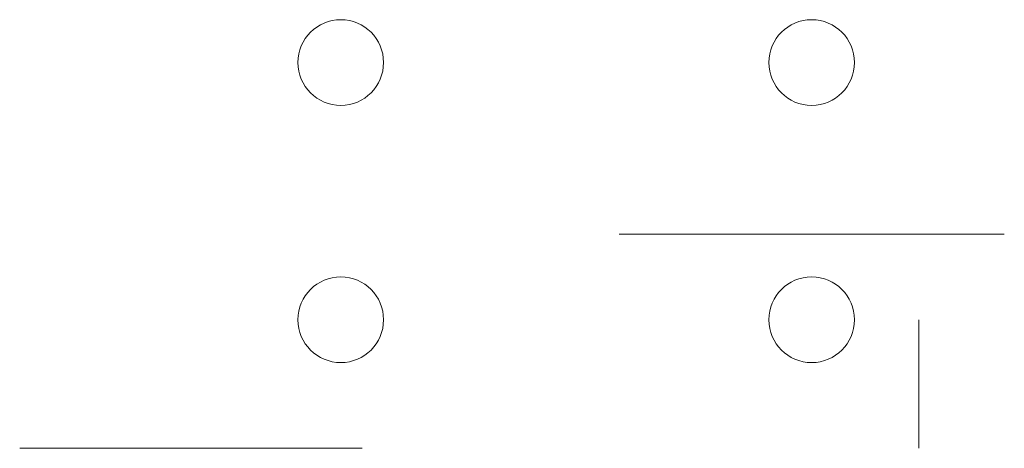
# Model space of a CAD drawing. Units: inches. Extents: x 1559 to 1674, y 0 to 50.
import ezdxf

# ---------------------------------------------------------------- set-up
doc = ezdxf.new("R2010")
doc.units = ezdxf.units.IN
doc.header["$MEASUREMENT"] = 0
doc.layers.add('M-CONS', color=8, linetype='Continuous', lineweight=13)

msp = doc.modelspace()

# ---------------------------------------------------------------- linework, layer by layer
at = {"layer": 'M-CONS'}
msp.add_line((1664.29, 0, 691.05), (1664.29, 15, 691.05), dxfattribs=at)
at = {"layer": 'M-CONS', "extrusion": (0, -1, 0), "elevation": -25}
msp.add_lwpolyline([(1674.29, 691.05), (1629.29, 771.05), (1629.29, 691.05)], close=True, dxfattribs=at)
at = {"layer": 'M-CONS'}
for centre in [(1596.79, 45, 691.05), (1651.79, 45, 691.05), (1596.79, 15, 691.05), (1651.79, 15, 691.05)]:
    msp.add_circle(centre, 5, dxfattribs=at)
at = {"layer": 'M-CONS', "extrusion": (0, -1, 0)}
msp.add_circle((1579.29, 806.05), 20, dxfattribs=at)

doc.saveas('drawing.dxf')
